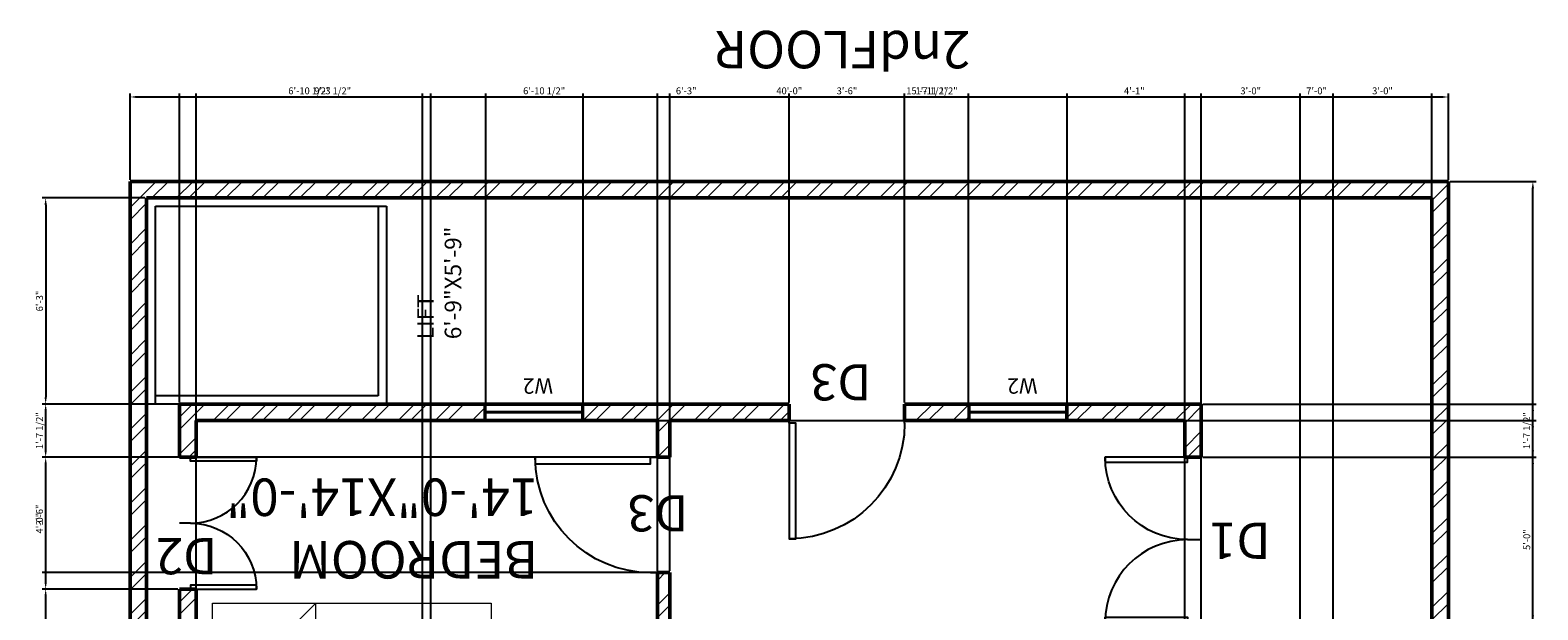
# Model space of a CAD drawing. Units: inches. Extents: x 244 to 2800, y 1060 to 1700.
# Tile 5 of 13: x 819 to 1368, y 1477 to 1688. Entities that reach past the tile are written whole.
import ezdxf

# ---------------------------------------------------------------- set-up
doc = ezdxf.new("R2010")
doc.units = ezdxf.units.IN
for name, color, linetype, lineweight in [('A-ANNO-DIMS', 2, 'Continuous', 18), ('A-ANNO-TEXT', 1, 'Continuous', 18), ('A-DOOR', 5, 'Continuous', 25), ('A-EQPM', 4, 'Continuous', 25), ('A-FURN', 9, 'Continuous', 18), ('A-GLAZ', 3, 'Continuous', 25), ('A-WALL', 7, 'Continuous', 50), ('A-WALL-PATT', 8, 'Continuous', 13)]:
    doc.layers.add(name, color=color, linetype=linetype, lineweight=lineweight)
doc.styles.get("Standard").update_dxf_attribs({"font": 'arial.ttf'})
doc.dimstyles.new('ISO-25', dxfattribs={"dimtxt": 2.5, "dimasz": 2.5, "dimexe": 1.25, "dimexo": 0.625, "dimtad": 1, "dimlunit": 4, "dimtxsty": 'Standard', "dimcen": 2.5, "dimadec": 0, "dimazin": 0, "dimtfac": 1, "dimtmove": 0, "dimatfit": 3, "dimfxl": 1, "dimarcsym": 0})

# ---------------------------------------------------------------- blocks, each defined once
blk = doc.blocks.new('*U2')
for p, q in [((0, 0), (0, -5)), ((30, 0), (30, -5))]:
    blk.add_line(p, q)
blk.add_lwpolyline([(0, 0), (0, 30), (1.75, 30), (1.75, 0)], close=True)
blk.add_arc((0, 0), 30, 0, 90)
blk = doc.blocks.new('Bed - Queen')
for p, q in [((0, -80.00003), (0, 0)), ((0, 0), (59.99999, 0)), ((59.99999, 0), (59.99999, -80.00003)), ((7.99999, -1.2), (28.79998, -1.2)), ((7.99999, -14.4), (7.99999, -1.2)), ((28.79998, -1.2), (28.79998, -14.4)), ((31.19999, -1.2), (51.99999, -1.2)), ((31.19999, -14.4), (31.19999, -1.2)), ((51.99999, -1.2), (51.99999, -16.4)), ((0, -14.4), (44.8, -14.4)), ((44.8, -16.8), (0, -16.8)), ((59.99999, -29.6), (44.8, -14.4)), ((44.8, -14.4), (44.8, -29.6)), ((51.99999, -16.4), (46.79936, -16.4)), ((44.8, -29.6), (59.99999, -29.6)), ((59.99999, -80.00003), (0, -80.00003))]:
    blk.add_line(p, q)
blk = doc.blocks.new('WIN-36')
for p, q in [((0, 0), (0, 6)), ((0, 6), (35.94, 6)), ((35.94, 6), (35.94, 0)), ((35.94, 0), (0, 0))]:
    blk.add_line(p, q)
blk = doc.blocks.new('LIFT-CAR')
for p, q in [((0, 0), (0, 72)), ((0, 72), (84, 72)), ((81, 72), (81, 3)), ((84, 72), (84, 0)), ((81, 3), (0, 3)), ((84, 0), (0, 0))]:
    blk.add_line(p, q)
blk = doc.blocks.new('*D107')
at = {"layer": 'A-ANNO-DIMS', "color": 0, "lineweight": -2, "transparency": 16777216}
for p, q in [((855.74, 1633.61), (855.74, 1664.99)), ((858.24, 1663.74), (1333.24, 1663.74)), ((1335.74, 1633.61), (1335.74, 1664.99))]:
    blk.add_line(p, q, dxfattribs=at)
at = {"layer": 'A-ANNO-DIMS', "color": 0, "transparency": 16777216}
for points in [[(858.24, 1664.15), (858.24, 1663.32), (855.74, 1663.74)], [(1333.24, 1664.15), (1333.24, 1663.32), (1335.74, 1663.74)]]:
    blk.add_solid(points, dxfattribs=at)
at = {"layer": 'Defpoints', "color": 0, "transparency": 16777216}
for p in [(1335.74, 1663.74), (855.74, 1632.99), (1335.74, 1632.99)]:
    blk.add_point(p, dxfattribs=at)
at = {"layer": 'A-ANNO-DIMS', "color": 0, "transparency": 16777216, "insert": (1095.74, 1665.64), "char_height": 2.5, "attachment_point": 5}
blk.add_mtext('40\'-0"', dxfattribs=at)
blk = doc.blocks.new('*D108')
at = {"layer": 'A-ANNO-DIMS', "color": 0, "lineweight": -2, "transparency": 16777216}
for p, q in [((1336.36, 1632.99), (1367.74, 1632.99)), ((1366.49, 1095.49), (1366.49, 1630.49)), ((1336.36, 1092.99), (1367.74, 1092.99))]:
    blk.add_line(p, q, dxfattribs=at)
at = {"layer": 'A-ANNO-DIMS', "color": 0, "transparency": 16777216}
for points in [[(1366.07, 1630.49), (1366.9, 1630.49), (1366.49, 1632.99)], [(1366.07, 1095.49), (1366.9, 1095.49), (1366.49, 1092.99)]]:
    blk.add_solid(points, dxfattribs=at)
at = {"layer": 'Defpoints', "color": 0, "transparency": 16777216}
for p in [(1335.74, 1632.99), (1366.49, 1632.99), (1335.74, 1092.99)]:
    blk.add_point(p, dxfattribs=at)
at = {"layer": 'A-ANNO-DIMS', "color": 0, "transparency": 16777216, "insert": (1364.58, 1362.99), "char_height": 2.5, "attachment_point": 5, "rotation": 90}
blk.add_mtext('45\'-0"', dxfattribs=at)
blk = doc.blocks.new('*D109')
at = {"layer": 'A-ANNO-DIMS', "color": 0, "lineweight": -2, "transparency": 16777216}
for p, q in [((861.11, 1626.99), (823.74, 1626.99)), ((824.99, 1624.49), (824.99, 1554.49)), ((873.11, 1551.99), (823.74, 1551.99))]:
    blk.add_line(p, q, dxfattribs=at)
at = {"layer": 'A-ANNO-DIMS', "color": 0, "transparency": 16777216}
for points in [[(824.57, 1624.49), (825.4, 1624.49), (824.99, 1626.99)], [(824.57, 1554.49), (825.4, 1554.49), (824.99, 1551.99)]]:
    blk.add_solid(points, dxfattribs=at)
at = {"layer": 'Defpoints', "color": 0, "transparency": 16777216}
for p in [(861.74, 1626.99), (824.99, 1551.99), (873.74, 1551.99)]:
    blk.add_point(p, dxfattribs=at)
at = {"layer": 'A-ANNO-DIMS', "color": 0, "transparency": 16777216, "insert": (823.08, 1589.49), "char_height": 2.5, "attachment_point": 5, "rotation": 90}
blk.add_mtext('6\'-3"', dxfattribs=at)
blk = doc.blocks.new('*D110')
at = {"layer": 'A-ANNO-DIMS', "color": 0, "lineweight": -2, "transparency": 16777216}
for p, q in [((1245.74, 1552.61), (1245.74, 1664.99)), ((1248.24, 1663.74), (1327.24, 1663.74)), ((1329.74, 1627.61), (1329.74, 1664.99))]:
    blk.add_line(p, q, dxfattribs=at)
at = {"layer": 'A-ANNO-DIMS', "color": 0, "transparency": 16777216}
for points in [[(1248.24, 1664.15), (1248.24, 1663.32), (1245.74, 1663.74)], [(1327.24, 1664.15), (1327.24, 1663.32), (1329.74, 1663.74)]]:
    blk.add_solid(points, dxfattribs=at)
at = {"layer": 'Defpoints', "color": 0, "transparency": 16777216}
for p in [(1329.74, 1663.74), (1329.74, 1626.99), (1245.74, 1551.99)]:
    blk.add_point(p, dxfattribs=at)
at = {"layer": 'A-ANNO-DIMS', "color": 0, "transparency": 16777216, "insert": (1287.74, 1665.64), "char_height": 2.5, "attachment_point": 5}
blk.add_mtext('7\'-0"', dxfattribs=at)
blk = doc.blocks.new('*D113')
at = {"layer": 'A-ANNO-DIMS', "color": 0, "lineweight": -2, "transparency": 16777216}
for p, q in [((873.74, 1552.61), (873.74, 1664.99)), ((876.24, 1663.74), (982.74, 1663.74)), ((985.24, 1552.61), (985.24, 1664.99))]:
    blk.add_line(p, q, dxfattribs=at)
at = {"layer": 'A-ANNO-DIMS', "color": 0, "transparency": 16777216}
for points in [[(876.24, 1664.15), (876.24, 1663.32), (873.74, 1663.74)], [(982.74, 1664.15), (982.74, 1663.32), (985.24, 1663.74)]]:
    blk.add_solid(points, dxfattribs=at)
at = {"layer": 'Defpoints', "color": 0, "transparency": 16777216}
for p in [(985.24, 1663.74), (873.74, 1551.99), (985.24, 1551.99)]:
    blk.add_point(p, dxfattribs=at)
at = {"layer": 'A-ANNO-DIMS', "color": 0, "transparency": 16777216, "insert": (929.49, 1665.65), "char_height": 2.5, "attachment_point": 5}
blk.add_mtext('9\'-3 1/2"', dxfattribs=at)
blk = doc.blocks.new('*D114')
at = {"layer": 'A-ANNO-DIMS', "color": 0, "lineweight": -2, "transparency": 16777216}
for p, q in [((1020.68, 1552.61), (1020.68, 1664.99)), ((1023.18, 1663.74), (1093.24, 1663.74)), ((1095.74, 1552.61), (1095.74, 1664.99))]:
    blk.add_line(p, q, dxfattribs=at)
at = {"layer": 'A-ANNO-DIMS', "color": 0, "transparency": 16777216}
for points in [[(1023.18, 1664.15), (1023.18, 1663.32), (1020.68, 1663.74)], [(1093.24, 1664.15), (1093.24, 1663.32), (1095.74, 1663.74)]]:
    blk.add_solid(points, dxfattribs=at)
at = {"layer": 'Defpoints', "color": 0, "transparency": 16777216}
for p in [(1095.74, 1663.74), (1020.68, 1551.99), (1095.74, 1551.99)]:
    blk.add_point(p, dxfattribs=at)
at = {"layer": 'A-ANNO-DIMS', "color": 0, "transparency": 16777216, "insert": (1058.21, 1665.64), "char_height": 2.5, "attachment_point": 5}
blk.add_mtext('6\'-3"', dxfattribs=at)
blk = doc.blocks.new('*D115')
at = {"layer": 'A-ANNO-DIMS', "color": 0, "lineweight": -2, "transparency": 16777216}
for p, q in [((1095.74, 1552.61), (1095.74, 1664.99)), ((1098.24, 1663.74), (1135.24, 1663.74)), ((1137.74, 1552.61), (1137.74, 1664.99))]:
    blk.add_line(p, q, dxfattribs=at)
at = {"layer": 'A-ANNO-DIMS', "color": 0, "transparency": 16777216}
for points in [[(1098.24, 1664.15), (1098.24, 1663.32), (1095.74, 1663.74)], [(1135.24, 1664.15), (1135.24, 1663.32), (1137.74, 1663.74)]]:
    blk.add_solid(points, dxfattribs=at)
at = {"layer": 'Defpoints', "color": 0, "transparency": 16777216}
for p in [(1137.74, 1663.74), (1095.74, 1551.99), (1137.74, 1551.99)]:
    blk.add_point(p, dxfattribs=at)
at = {"layer": 'A-ANNO-DIMS', "color": 0, "transparency": 16777216, "insert": (1116.74, 1665.64), "char_height": 2.5, "attachment_point": 5}
blk.add_mtext('3\'-6"', dxfattribs=at)
blk = doc.blocks.new('*D116')
at = {"layer": 'A-ANNO-DIMS', "color": 0, "lineweight": -2, "transparency": 16777216}
for p, q in [((1137.74, 1552.61), (1137.74, 1664.99)), ((1140.24, 1663.74), (1158.54, 1663.74)), ((1161.04, 1552.61), (1161.04, 1664.99))]:
    blk.add_line(p, q, dxfattribs=at)
at = {"layer": 'A-ANNO-DIMS', "color": 0, "transparency": 16777216}
for points in [[(1140.24, 1664.15), (1140.24, 1663.32), (1137.74, 1663.74)], [(1158.54, 1664.15), (1158.54, 1663.32), (1161.04, 1663.74)]]:
    blk.add_solid(points, dxfattribs=at)
at = {"layer": 'Defpoints', "color": 0, "transparency": 16777216}
for p in [(1161.04, 1663.74), (1137.74, 1551.99), (1161.04, 1551.99)]:
    blk.add_point(p, dxfattribs=at)
at = {"layer": 'A-ANNO-DIMS', "color": 0, "transparency": 16777216, "insert": (1149.39, 1665.65), "char_height": 2.5, "attachment_point": 5}
blk.add_mtext('1\'-11 1/2"', dxfattribs=at)
blk = doc.blocks.new('*D117')
at = {"layer": 'A-ANNO-DIMS', "color": 0, "lineweight": -2, "transparency": 16777216}
for p, q in [((1196.98, 1552.61), (1196.98, 1664.99)), ((1199.48, 1663.74), (1243.24, 1663.74)), ((1245.74, 1552.61), (1245.74, 1664.99))]:
    blk.add_line(p, q, dxfattribs=at)
at = {"layer": 'A-ANNO-DIMS', "color": 0, "transparency": 16777216}
for points in [[(1199.48, 1664.15), (1199.48, 1663.32), (1196.98, 1663.74)], [(1243.24, 1664.15), (1243.24, 1663.32), (1245.74, 1663.74)]]:
    blk.add_solid(points, dxfattribs=at)
at = {"layer": 'Defpoints', "color": 0, "transparency": 16777216}
for p in [(1245.74, 1663.74), (1196.98, 1551.99), (1245.74, 1551.99)]:
    blk.add_point(p, dxfattribs=at)
at = {"layer": 'A-ANNO-DIMS', "color": 0, "transparency": 16777216, "insert": (1221.36, 1665.62), "char_height": 2.5, "attachment_point": 5}
blk.add_mtext('4\'-1"', dxfattribs=at)
blk = doc.blocks.new('*D120')
at = {"layer": 'A-ANNO-DIMS', "color": 0, "lineweight": -2, "transparency": 16777216}
for p, q in [((873.11, 1484.64), (823.74, 1484.64)), ((824.99, 1349.76), (824.99, 1482.14)), ((873.11, 1347.26), (823.74, 1347.26))]:
    blk.add_line(p, q, dxfattribs=at)
at = {"layer": 'A-ANNO-DIMS', "color": 0, "transparency": 16777216}
for points in [[(824.57, 1482.14), (825.4, 1482.14), (824.99, 1484.64)], [(824.57, 1349.76), (825.4, 1349.76), (824.99, 1347.26)]]:
    blk.add_solid(points, dxfattribs=at)
at = {"layer": 'Defpoints', "color": 0, "transparency": 16777216}
for p in [(824.99, 1484.64), (873.74, 1484.64), (873.74, 1347.26)]:
    blk.add_point(p, dxfattribs=at)
at = {"layer": 'A-ANNO-DIMS', "color": 0, "transparency": 16777216, "insert": (823.07, 1415.95), "char_height": 2.5, "attachment_point": 5, "rotation": 90}
blk.add_mtext('11\'-5 1/2"', dxfattribs=at)
blk = doc.blocks.new('*D121')
at = {"layer": 'A-ANNO-DIMS', "color": 0, "lineweight": -2, "transparency": 16777216}
for p, q in [((873.11, 1532.64), (823.74, 1532.64)), ((824.99, 1487.14), (824.99, 1530.14)), ((873.11, 1484.64), (823.74, 1484.64))]:
    blk.add_line(p, q, dxfattribs=at)
at = {"layer": 'A-ANNO-DIMS', "color": 0, "transparency": 16777216}
for points in [[(824.57, 1530.14), (825.4, 1530.14), (824.99, 1532.64)], [(824.57, 1487.14), (825.4, 1487.14), (824.99, 1484.64)]]:
    blk.add_solid(points, dxfattribs=at)
at = {"layer": 'Defpoints', "color": 0, "transparency": 16777216}
for p in [(824.99, 1532.64), (873.74, 1532.64), (873.74, 1484.64)]:
    blk.add_point(p, dxfattribs=at)
at = {"layer": 'A-ANNO-DIMS', "color": 0, "transparency": 16777216, "insert": (823.08, 1508.64), "char_height": 2.5, "attachment_point": 5, "rotation": 90}
blk.add_mtext('4\'-0"', dxfattribs=at)
blk = doc.blocks.new('*D122')
at = {"layer": 'A-ANNO-DIMS', "color": 0, "lineweight": -2, "transparency": 16777216}
for p, q in [((873.11, 1551.99), (823.74, 1551.99)), ((824.99, 1535.14), (824.99, 1549.49)), ((873.11, 1532.64), (823.74, 1532.64))]:
    blk.add_line(p, q, dxfattribs=at)
at = {"layer": 'A-ANNO-DIMS', "color": 0, "transparency": 16777216}
for points in [[(824.57, 1549.49), (825.4, 1549.49), (824.99, 1551.99)], [(824.57, 1535.14), (825.4, 1535.14), (824.99, 1532.64)]]:
    blk.add_solid(points, dxfattribs=at)
at = {"layer": 'Defpoints', "color": 0, "transparency": 16777216}
for p in [(824.99, 1551.99), (873.74, 1551.99), (873.74, 1532.64)]:
    blk.add_point(p, dxfattribs=at)
at = {"layer": 'A-ANNO-DIMS', "color": 0, "transparency": 16777216, "insert": (823.07, 1542.31), "char_height": 2.5, "attachment_point": 5, "rotation": 90}
blk.add_mtext('1\'-7 1/2"', dxfattribs=at)
blk = doc.blocks.new('*D125')
at = {"layer": 'A-ANNO-DIMS', "color": 0, "lineweight": -2, "transparency": 16777216}
for p, q in [((880.36, 1545.99), (1367.74, 1545.99)), ((1366.49, 1375.49), (1366.49, 1543.49)), ((880.36, 1372.99), (1367.74, 1372.99))]:
    blk.add_line(p, q, dxfattribs=at)
at = {"layer": 'A-ANNO-DIMS', "color": 0, "transparency": 16777216}
for points in [[(1366.07, 1543.49), (1366.9, 1543.49), (1366.49, 1545.99)], [(1366.07, 1375.49), (1366.9, 1375.49), (1366.49, 1372.99)]]:
    blk.add_solid(points, dxfattribs=at)
at = {"layer": 'Defpoints', "color": 0, "transparency": 16777216}
for p in [(879.74, 1545.99), (1366.49, 1545.99), (879.74, 1372.99)]:
    blk.add_point(p, dxfattribs=at)
at = {"layer": 'A-ANNO-DIMS', "color": 0, "transparency": 16777216, "insert": (1364.58, 1459.49), "char_height": 2.5, "attachment_point": 5, "rotation": 90}
blk.add_mtext('14\'-5"', dxfattribs=at)
blk = doc.blocks.new('*D126')
at = {"layer": 'A-ANNO-DIMS', "color": 0, "lineweight": -2, "transparency": 16777216}
for p, q in [((879.74, 1373.61), (879.74, 1664.99)), ((882.24, 1663.74), (959.74, 1663.74)), ((962.24, 1369.11), (962.24, 1664.99))]:
    blk.add_line(p, q, dxfattribs=at)
at = {"layer": 'A-ANNO-DIMS', "color": 0, "transparency": 16777216}
for points in [[(882.24, 1664.15), (882.24, 1663.32), (879.74, 1663.74)], [(959.74, 1664.15), (959.74, 1663.32), (962.24, 1663.74)]]:
    blk.add_solid(points, dxfattribs=at)
at = {"layer": 'Defpoints', "color": 0, "transparency": 16777216}
for p in [(962.24, 1663.74), (879.74, 1372.99), (962.24, 1368.49)]:
    blk.add_point(p, dxfattribs=at)
at = {"layer": 'A-ANNO-DIMS', "color": 0, "transparency": 16777216, "insert": (920.99, 1665.65), "char_height": 2.5, "attachment_point": 5}
blk.add_mtext('6\'-10 1/2"', dxfattribs=at)
blk = doc.blocks.new('*D127')
at = {"layer": 'A-ANNO-DIMS', "color": 0, "lineweight": -2, "transparency": 16777216}
for p, q in [((965.24, 1369.11), (965.24, 1664.99)), ((967.74, 1663.74), (1045.24, 1663.74)), ((1047.74, 1373.61), (1047.74, 1664.99))]:
    blk.add_line(p, q, dxfattribs=at)
at = {"layer": 'A-ANNO-DIMS', "color": 0, "transparency": 16777216}
for points in [[(967.74, 1664.15), (967.74, 1663.32), (965.24, 1663.74)], [(1045.24, 1664.15), (1045.24, 1663.32), (1047.74, 1663.74)]]:
    blk.add_solid(points, dxfattribs=at)
at = {"layer": 'Defpoints', "color": 0, "transparency": 16777216}
for p in [(1047.74, 1663.74), (1047.74, 1372.99), (965.24, 1368.49)]:
    blk.add_point(p, dxfattribs=at)
at = {"layer": 'A-ANNO-DIMS', "color": 0, "transparency": 16777216, "insert": (1006.49, 1665.65), "char_height": 2.5, "attachment_point": 5}
blk.add_mtext('6\'-10 1/2"', dxfattribs=at)
blk = doc.blocks.new('*D138')
at = {"layer": 'A-ANNO-DIMS', "color": 0, "lineweight": -2, "transparency": 16777216}
for p, q in [((1047.11, 1532.64), (823.74, 1532.64)), ((824.99, 1493.14), (824.99, 1530.14)), ((1047.11, 1490.64), (823.74, 1490.64))]:
    blk.add_line(p, q, dxfattribs=at)
at = {"layer": 'A-ANNO-DIMS', "color": 0, "transparency": 16777216}
for points in [[(824.57, 1530.14), (825.4, 1530.14), (824.99, 1532.64)], [(824.57, 1493.14), (825.4, 1493.14), (824.99, 1490.64)]]:
    blk.add_solid(points, dxfattribs=at)
at = {"layer": 'Defpoints', "color": 0, "transparency": 16777216}
for p in [(824.99, 1532.64), (1047.74, 1532.64), (1047.74, 1490.64)]:
    blk.add_point(p, dxfattribs=at)
at = {"layer": 'A-ANNO-DIMS', "color": 0, "transparency": 16777216, "insert": (823.08, 1511.64), "char_height": 2.5, "attachment_point": 5, "rotation": 90}
blk.add_mtext('3\'-6"', dxfattribs=at)
blk = doc.blocks.new('*D141')
at = {"layer": 'A-ANNO-DIMS', "color": 0, "lineweight": -2, "transparency": 16777216}
for p, q in [((1246.36, 1532.64), (1367.74, 1532.64)), ((1366.49, 1475.14), (1366.49, 1530.14)), ((1246.36, 1472.64), (1367.74, 1472.64))]:
    blk.add_line(p, q, dxfattribs=at)
at = {"layer": 'A-ANNO-DIMS', "color": 0, "transparency": 16777216}
for points in [[(1366.07, 1530.14), (1366.9, 1530.14), (1366.49, 1532.64)], [(1366.07, 1475.14), (1366.9, 1475.14), (1366.49, 1472.64)]]:
    blk.add_solid(points, dxfattribs=at)
at = {"layer": 'Defpoints', "color": 0, "transparency": 16777216}
for p in [(1245.74, 1532.64), (1366.49, 1532.64), (1245.74, 1472.64)]:
    blk.add_point(p, dxfattribs=at)
at = {"layer": 'A-ANNO-DIMS', "color": 0, "transparency": 16777216, "insert": (1364.58, 1502.64), "char_height": 2.5, "attachment_point": 5, "rotation": 90}
blk.add_mtext('5\'-0"', dxfattribs=at)
blk = doc.blocks.new('*D142')
at = {"layer": 'A-ANNO-DIMS', "color": 0, "lineweight": -2, "transparency": 16777216}
for p, q in [((1246.36, 1551.99), (1367.74, 1551.99)), ((1366.49, 1535.14), (1366.49, 1549.49)), ((1246.36, 1532.64), (1367.74, 1532.64))]:
    blk.add_line(p, q, dxfattribs=at)
at = {"layer": 'A-ANNO-DIMS', "color": 0, "transparency": 16777216}
for points in [[(1366.07, 1549.49), (1366.9, 1549.49), (1366.49, 1551.99)], [(1366.07, 1535.14), (1366.9, 1535.14), (1366.49, 1532.64)]]:
    blk.add_solid(points, dxfattribs=at)
at = {"layer": 'Defpoints', "color": 0, "transparency": 16777216}
for p in [(1245.74, 1551.99), (1366.49, 1551.99), (1245.74, 1532.64)]:
    blk.add_point(p, dxfattribs=at)
at = {"layer": 'A-ANNO-DIMS', "color": 0, "transparency": 16777216, "insert": (1364.57, 1542.31), "char_height": 2.5, "attachment_point": 5, "rotation": 90}
blk.add_mtext('1\'-7 1/2"', dxfattribs=at)
blk = doc.blocks.new('*D145')
at = {"layer": 'A-ANNO-DIMS', "color": 0, "lineweight": -2, "transparency": 16777216}
for p, q in [((1245.74, 1243.61), (1245.74, 1664.99)), ((1248.24, 1663.74), (1279.24, 1663.74)), ((1281.74, 1243.61), (1281.74, 1664.99))]:
    blk.add_line(p, q, dxfattribs=at)
at = {"layer": 'A-ANNO-DIMS', "color": 0, "transparency": 16777216}
for points in [[(1248.24, 1664.15), (1248.24, 1663.32), (1245.74, 1663.74)], [(1279.24, 1664.15), (1279.24, 1663.32), (1281.74, 1663.74)]]:
    blk.add_solid(points, dxfattribs=at)
at = {"layer": 'Defpoints', "color": 0, "transparency": 16777216}
for p in [(1281.74, 1663.74), (1245.74, 1242.99), (1281.74, 1242.99)]:
    blk.add_point(p, dxfattribs=at)
at = {"layer": 'A-ANNO-DIMS', "color": 0, "transparency": 16777216, "insert": (1263.74, 1665.64), "char_height": 2.5, "attachment_point": 5}
blk.add_mtext('3\'-0"', dxfattribs=at)
blk = doc.blocks.new('*D146')
at = {"layer": 'A-ANNO-DIMS', "color": 0, "lineweight": -2, "transparency": 16777216}
for p, q in [((1293.74, 1243.61), (1293.74, 1664.99)), ((1296.24, 1663.74), (1327.24, 1663.74)), ((1329.74, 1243.61), (1329.74, 1664.99))]:
    blk.add_line(p, q, dxfattribs=at)
at = {"layer": 'A-ANNO-DIMS', "color": 0, "transparency": 16777216}
for points in [[(1296.24, 1664.15), (1296.24, 1663.32), (1293.74, 1663.74)], [(1327.24, 1664.15), (1327.24, 1663.32), (1329.74, 1663.74)]]:
    blk.add_solid(points, dxfattribs=at)
at = {"layer": 'Defpoints', "color": 0, "transparency": 16777216}
for p in [(1329.74, 1663.74), (1293.74, 1242.99), (1329.74, 1242.99)]:
    blk.add_point(p, dxfattribs=at)
at = {"layer": 'A-ANNO-DIMS', "color": 0, "transparency": 16777216, "insert": (1311.74, 1665.64), "char_height": 2.5, "attachment_point": 5}
blk.add_mtext('3\'-0"', dxfattribs=at)
blk = doc.blocks.new('*D147')
at = {"layer": 'A-ANNO-DIMS', "color": 0, "lineweight": -2, "transparency": 16777216}
for p, q in [((1052.24, 1491.26), (1052.24, 1664.99)), ((1054.74, 1663.74), (1237.24, 1663.74)), ((1239.74, 1473.26), (1239.74, 1664.99))]:
    blk.add_line(p, q, dxfattribs=at)
at = {"layer": 'A-ANNO-DIMS', "color": 0, "transparency": 16777216}
for points in [[(1054.74, 1664.15), (1054.74, 1663.32), (1052.24, 1663.74)], [(1237.24, 1664.15), (1237.24, 1663.32), (1239.74, 1663.74)]]:
    blk.add_solid(points, dxfattribs=at)
at = {"layer": 'Defpoints', "color": 0, "transparency": 16777216}
for p in [(1239.74, 1663.74), (1052.24, 1490.64), (1239.74, 1472.64)]:
    blk.add_point(p, dxfattribs=at)
at = {"layer": 'A-ANNO-DIMS', "color": 0, "transparency": 16777216, "insert": (1145.99, 1665.65), "char_height": 2.5, "attachment_point": 5}
blk.add_mtext('15\'-7 1/2"', dxfattribs=at)

msp = doc.modelspace()

# ---------------------------------------------------------------- hatches: boundary and pattern name
at = {"layer": 'A-WALL-PATT'}
h = msp.add_hatch(dxfattribs=at)
h.set_pattern_fill('ANSI32', color=256)
h.paths.add_polyline_path([(1335.736, 1632.986), (855.736, 1632.986), (855.736, 1092.986), (1335.736, 1092.986)])
h.paths.add_polyline_path([(1329.736, 1626.986), (1329.736, 1098.986), (1245.736, 1098.986), (861.736, 1098.986), (861.736, 1626.986)], flags=16)
h.paths.add_polyline_path([(1245.736, 1551.986), (1245.736, 1532.64), (1239.736, 1532.64), (1239.736, 1545.986), (1137.736, 1545.986), (1137.736, 1551.986)], flags=0)
h.paths.add_polyline_path([(1196.984, 1551.986), (1196.984, 1545.986), (1161.039, 1545.986), (1161.039, 1551.986)], flags=0)
h.paths.add_polyline_path([(1196.484, 1548.786), (1161.539, 1548.786), (1161.539, 1549.186), (1196.484, 1549.186)], flags=0)
h.paths.add_polyline_path([(1245.736, 1472.64), (1245.736, 1242.986), (1281.736, 1242.986), (1281.736, 1134.986), (1293.736, 1134.986), (1293.736, 1242.986), (1329.736, 1242.986), (1329.736, 1134.986), (1245.736, 1134.986), (1245.736, 1110.986), (1139.236, 1110.986), (873.736, 1110.986), (873.736, 1484.64), (879.736, 1484.64), (879.736, 1372.986), (1014.736, 1372.986), (1014.736, 1368.486), (965.236, 1368.486), (965.236, 1296.486), (1047.736, 1296.486), (1047.736, 1368.486), (1044.736, 1368.486), (1044.736, 1372.986), (1047.736, 1372.986), (1047.736, 1490.64), (1052.236, 1490.64), (1052.236, 1288.986), (1047.736, 1288.986), (1047.736, 1291.986), (912.736, 1291.986), (912.736, 1296.486), (962.236, 1296.486), (962.236, 1368.486), (879.736, 1368.486), (879.736, 1296.486), (882.736, 1296.486), (882.736, 1291.986), (879.736, 1291.986), (879.736, 1116.986), (1047.736, 1116.986), (1047.736, 1246.986), (1052.236, 1246.986), (1052.236, 1116.986), (1088.236, 1116.986), (1088.236, 1152.986), (1088.236, 1313.486), (1095.736, 1313.486), (1095.736, 1308.986), (1092.736, 1308.986), (1092.736, 1157.486), (1128.736, 1157.486), (1128.736, 1116.986), (1139.236, 1116.986), (1175.181, 1116.986), (1239.736, 1116.986), (1239.736, 1308.986), (1137.736, 1308.986), (1137.736, 1313.486), (1239.736, 1313.486), (1239.736, 1472.64)], flags=0)
h.paths.add_polyline_path([(1245.736, 1462.542), (1245.736, 1414.597), (1239.736, 1414.597), (1239.736, 1462.542)], flags=0)
h.paths.add_polyline_path([(1242.936, 1462.042), (1242.936, 1415.097), (1242.536, 1415.097), (1242.536, 1462.042)], flags=0)
h.paths.add_polyline_path([(1095.736, 1551.986), (1095.736, 1545.986), (1052.236, 1545.986), (1052.236, 1532.64), (1047.736, 1532.64), (1047.736, 1545.986), (879.736, 1545.986), (879.736, 1532.64), (873.736, 1532.64), (873.736, 1551.986), (865.04, 1551.986), (865.04, 1623.986), (949.04, 1623.986), (949.04, 1551.986)], flags=0)
h.paths.add_polyline_path([(1020.681, 1551.986), (1020.681, 1545.986), (984.736, 1545.986), (984.736, 1551.986)], flags=0)
h.paths.add_polyline_path([(1020.181, 1548.786), (985.236, 1548.786), (985.236, 1549.186), (1020.181, 1549.186)], flags=0)
h.paths.add_polyline_path([(879.736, 1347.762), (879.736, 1323.817), (873.736, 1323.817), (873.736, 1347.762)], flags=0)
h.paths.add_polyline_path([(876.936, 1347.262), (876.936, 1324.317), (876.536, 1324.317), (876.536, 1347.262)], flags=0)
h.paths.add_polyline_path([(1124.236, 1152.986), (1124.236, 1116.986), (1088.236, 1116.986), (1088.236, 1152.986)], flags=0)
h.paths.add_polyline_path([(879.736, 1287.983), (879.736, 1252.038), (873.736, 1252.038), (873.736, 1287.983)], flags=0)
h.paths.add_polyline_path([(876.936, 1287.483), (876.936, 1252.538), (876.536, 1252.538), (876.536, 1287.483)], flags=0)
h.paths.add_polyline_path([(1175.181, 1116.986), (1175.181, 1110.986), (1139.236, 1110.986), (1139.236, 1114.186), (1174.681, 1114.186), (1174.681, 1116.986)], flags=0)
h.paths.add_polyline_path([(1040.103, 1116.986), (1040.103, 1110.986), (1004.158, 1110.986), (1004.158, 1116.986)], flags=0)
h.paths.add_polyline_path([(1039.603, 1113.786), (1004.658, 1113.786), (1004.658, 1114.186), (1039.603, 1114.186)], flags=0)
h.paths.add_polyline_path([(1164.972, 1113.308), (1150.368, 1113.308), (1150.368, 1101.713), (1164.972, 1101.713)], flags=8)
h.paths.add_polyline_path([(1033.179, 1112.552), (1018.576, 1112.552), (1018.576, 1100.958), (1033.179, 1100.958)], flags=8)
h.paths.add_polyline_path([(874.571, 1270.316), (859.967, 1270.316), (859.967, 1258.722), (874.571, 1258.722)], flags=24)
h.paths.add_polyline_path([(1011.225, 1564.465), (996.622, 1564.465), (996.622, 1552.871), (1011.225, 1552.871)], flags=8)
h.paths.add_polyline_path([(1187.63, 1564.482), (1173.026, 1564.482), (1173.026, 1552.887), (1187.63, 1552.887)], flags=8)
h.paths.add_polyline_path([(1259.132, 1444.47), (1244.529, 1444.47), (1244.529, 1432.875), (1259.132, 1432.875)], flags=8)
h.paths.add_polyline_path([(875.239, 1344.511), (860.635, 1344.511), (860.635, 1332.916), (875.239, 1332.916)], flags=24)
h.paths.add_polyline_path([(892.18, 1510.489), (862.03, 1510.489), (862.03, 1483.307), (892.18, 1483.307)], flags=8)
h.paths.add_polyline_path([(912.199, 1310.068), (882.049, 1310.068), (882.049, 1282.887), (912.199, 1282.887)], flags=8)
h.paths.add_polyline_path([(1043.03, 1389.229), (1012.88, 1389.229), (1012.88, 1362.047), (1043.03, 1362.047)], flags=8)
h.paths.add_polyline_path([(1058.3, 1285.41), (1028.149, 1285.41), (1028.149, 1258.229), (1058.3, 1258.229)], flags=8)
h.paths.add_polyline_path([(1129.051, 1325.331), (1098.901, 1325.331), (1098.901, 1298.15), (1129.051, 1298.15)], flags=8)
h.paths.add_polyline_path([(1063.761, 1526.078), (1033.611, 1526.078), (1033.611, 1498.897), (1063.761, 1498.897)], flags=8)
h.paths.add_polyline_path([(1130.374, 1573.756), (1100.224, 1573.756), (1100.224, 1546.575), (1130.374, 1546.575)], flags=8)
h.paths.add_polyline_path([(1275.672, 1516.103), (1245.522, 1516.103), (1245.522, 1488.922), (1275.672, 1488.922)], flags=8)
h.paths.add_polyline_path([(979.613, 1573.477), (979.613, 1615.869), (957.159, 1615.869), (957.159, 1573.477)], flags=8)
h.paths.add_polyline_path([(1311.481, 1266.003), (1254.484, 1266.003), (1254.484, 1252.05), (1311.481, 1252.05)], flags=8)
h.paths.add_polyline_path([(1159.757, 1266.713), (1159.757, 1153.038), (1197.594, 1153.038), (1197.594, 1266.713)], flags=8)
h.paths.add_polyline_path([(1139.055, 1456.095), (1139.055, 1323.863), (1184.409, 1323.863), (1184.409, 1456.095)], flags=8)
h.paths.add_polyline_path([(936.318, 1364.302), (878.595, 1364.302), (878.595, 1333.511), (936.318, 1333.511)], flags=8)
h.paths.add_polyline_path([(1042.961, 1335.109), (985.238, 1335.109), (985.238, 1304.318), (1042.961, 1304.318)], flags=8)
h.paths.add_polyline_path([(1002.135, 1273.839), (885.452, 1273.839), (885.452, 1222.91), (1002.135, 1222.91)], flags=8)
h.paths.add_polyline_path([(1009.771, 1532.646), (893.088, 1532.646), (893.088, 1481.717), (1009.771, 1481.717)], flags=8)
h = msp.add_hatch(dxfattribs=at)
h.set_pattern_fill('ANSI32', color=256)
h.paths.add_polyline_path([(984.736, 1551.986), (873.736, 1551.986), (873.736, 1532.64), (877.736, 1532.64), (879.736, 1532.64), (879.736, 1545.986), (984.736, 1545.986)])
h = msp.add_hatch(dxfattribs=at)
h.set_pattern_fill('ANSI32', color=256)
h.paths.add_polyline_path([(1095.736, 1551.986), (1055.236, 1551.986), (1020.681, 1551.986), (1020.681, 1545.986), (1047.736, 1545.986), (1047.736, 1532.64), (1052.236, 1532.64), (1052.236, 1545.986), (1055.236, 1545.986), (1095.736, 1545.986)])
h = msp.add_hatch(dxfattribs=at)
h.set_pattern_fill('ANSI32', color=256)
h.paths.add_polyline_path([(1161.039, 1551.986), (1137.736, 1551.986), (1137.736, 1545.986), (1161.039, 1545.986)])
h = msp.add_hatch(dxfattribs=at)
h.set_pattern_fill('ANSI32', color=256)
h.paths.add_polyline_path([(1245.736, 1551.986), (1196.984, 1551.986), (1196.984, 1545.986), (1239.736, 1545.986), (1239.736, 1532.64), (1245.736, 1532.64)])
h = msp.add_hatch(dxfattribs=at)
h.set_pattern_fill('ANSI32', color=256)
h.paths.add_polyline_path([(1052.236, 1490.64), (1047.736, 1490.64), (1047.736, 1372.986), (1044.736, 1372.986), (1044.736, 1368.486), (1047.736, 1368.486), (1047.736, 1296.486), (965.236, 1296.486), (965.236, 1368.486), (1014.736, 1368.486), (1014.736, 1372.986), (879.736, 1372.986), (879.736, 1484.64), (877.736, 1484.64), (873.736, 1484.64), (873.736, 1347.762), (879.736, 1347.762), (879.736, 1368.486), (962.236, 1368.486), (962.236, 1296.486), (912.736, 1296.486), (912.736, 1291.986), (915.736, 1291.986), (1047.736, 1291.986), (1047.736, 1288.986), (1052.236, 1288.986)])

# ---------------------------------------------------------------- linework, layer by layer
at = {"layer": 'A-GLAZ'}
for p, q in [((985.236, 1545.986), (985.236, 1551.986)), ((1020.181, 1549.186), (985.236, 1549.186)), ((1020.181, 1548.786), (985.236, 1548.786)), ((1020.181, 1551.986), (1020.181, 1545.986)), ((1161.539, 1545.986), (1161.539, 1551.986)), ((1196.484, 1549.186), (1161.539, 1549.186)), ((1196.484, 1548.786), (1161.539, 1548.786)), ((1196.484, 1551.986), (1196.484, 1545.986))]:
    msp.add_line(p, q, dxfattribs=at)
at = {"layer": 'A-WALL'}
for p, q in [((1335.736, 1632.986), (855.736, 1632.986)), ((855.736, 1632.986), (855.736, 1092.986)), ((1335.736, 1092.986), (1335.736, 1632.986)), ((1329.736, 1626.986), (861.736, 1626.986)), ((861.736, 1626.986), (861.736, 1098.986)), ((1329.736, 1098.986), (1329.736, 1626.986)), ((873.736, 1551.986), (873.736, 1532.64)), ((873.736, 1551.986), (1095.736, 1551.986)), ((1055.236, 1551.986), (1095.736, 1551.986)), ((1095.736, 1545.986), (1095.736, 1551.986)), ((1137.736, 1551.986), (1245.736, 1551.986)), ((1137.736, 1551.986), (1137.736, 1545.986)), ((1245.736, 1532.64), (1245.736, 1551.986)), ((879.736, 1545.986), (879.736, 1532.64)), ((879.736, 1545.986), (1047.736, 1545.986)), ((1047.736, 1545.986), (1047.736, 1532.64)), ((1052.236, 1545.986), (1052.236, 1532.64)), ((1052.236, 1545.986), (1095.736, 1545.986)), ((1052.236, 1545.986), (1055.236, 1545.986)), ((1137.736, 1545.986), (1239.736, 1545.986)), ((1239.736, 1532.64), (1239.736, 1545.986)), ((879.736, 1532.64), (873.736, 1532.64)), ((1052.236, 1532.64), (1047.736, 1532.64)), ((1239.657, 1532.64), (1245.736, 1532.64)), ((1047.736, 1490.64), (1047.736, 1372.986)), ((1047.736, 1490.64), (1052.236, 1490.64)), ((1052.236, 1490.64), (1052.236, 1288.986)), ((873.736, 1484.64), (879.736, 1484.64)), ((873.736, 1484.64), (873.736, 1110.986)), ((879.736, 1484.64), (879.736, 1372.986))]:
    msp.add_line(p, q, dxfattribs=at)

# ---------------------------------------------------------------- block references
at = {"layer": 'A-DOOR'}
for p, xscale, yscale, zscale, rotation in [((1095.736, 1544.986), -1.399999999999999, 1.399999999999999, 1.399999999999999, 180), ((877.736, 1532.64), 0.8000000000000049, 0.8000000000000049, 0.8000000000000049, 270), ((1045.236, 1532.64), -1.399999999999999, 1.399999999999999, 1.399999999999999, 90), ((1240.736, 1532.64), -0.9999956819955501, 0.9999956819955501, 0.9999956819955501, 90), ((877.736, 1484.64), -0.8000000000000049, 0.8000000000000049, 0.8000000000000049, 270), ((1240.736, 1472.64), 0.9999956819955501, 0.9999956819955501, 0.9999956819955501, 90)]:
    msp.add_blockref('*U2', p, dxfattribs=dict(at, xscale=xscale, yscale=yscale, zscale=zscale, rotation=rotation))
at = {"layer": 'A-EQPM'}
msp.add_blockref('LIFT-CAR', (865.04, 1551.986), dxfattribs=at)
at = {"layer": 'A-FURN', "xscale": 1.268227082860182, "yscale": 1.268227082860182, "zscale": 1.268227082860182, "rotation": 90}
msp.add_blockref('Bed - Queen', (885.782, 1403.45), dxfattribs=at)
at = {"layer": 'A-GLAZ', "rotation": 180}
for p in [(1020.681, 1551.986), (1196.984, 1551.986)]:
    msp.add_blockref('WIN-36', p, dxfattribs=at)

# ---------------------------------------------------------------- texts
at = {"layer": 'A-ANNO-TEXT', "attachment_point": 1}
for s, width, gutter_width, insert, char_height, rotation in [('2ndFLOOR', 25.27039, 68.243, (1161.668, 1674.165), 13.6485, 180), ('LIFT\\P6\'-9"X5\'-9"', 12.02436, 30.086, (960.256, 1575.597), 6.01727, 90), ('D3', 20.58737, 65.951, (1125.655, 1553.309), 13.1902, 180), ('W2', 2.91536, 28.132, (1009.723, 1555.743), 5.6265, 180), ('W2', 2.91536, 28.132, (1186.127, 1555.76), 5.6265, 180), ('BEDROOM\\P14\'-0"X14\'-0"', 25.27039, 68.243, (1004.282, 1488.499), 13.64851, 180), ('D3', 20.58737, 65.951, (1059.042, 1505.631), 13.1902, 180), ('D1', 20.58737, 65.951, (1270.953, 1495.656), 13.1902, 180), ('D2', 20.58737, 65.951, (887.461, 1490.042), 13.1902, 180)]:
    msp.add_mtext_dynamic_manual_height_columns(s, width=width, gutter_width=gutter_width, heights=[0], dxfattribs=dict(at, insert=insert, char_height=char_height, rotation=rotation))

# ---------------------------------------------------------------- dimensions: what is measured, and where the dimension line sits
at = {"layer": 'A-ANNO-DIMS'}
for base, p1, p2, picture, middle in [((985.236, 1663.736), (873.736, 1551.986), (985.236, 1551.986), '*D113', (929.486, 1665.655)), ((962.236, 1663.736), (879.736, 1372.986), (962.236, 1368.486), '*D126', (920.986, 1665.654)), ((1047.736, 1663.736), (965.236, 1368.486), (1047.736, 1372.986), '*D127', (1006.486, 1665.654)), ((1239.736, 1663.736), (1052.236, 1490.64), (1239.736, 1472.64), '*D147', (1145.986, 1665.654)), ((1161.039, 1663.736), (1137.736, 1551.986), (1161.039, 1551.986), '*D116', (1149.388, 1665.654)), ((1335.736, 1663.736), (855.736, 1632.986), (1335.736, 1632.986), '*D107', (1095.736, 1665.638)), ((1095.736, 1663.736), (1020.681, 1551.986), (1095.736, 1551.986), '*D114', (1058.208, 1665.638)), ((1137.736, 1663.736), (1095.736, 1551.986), (1137.736, 1551.986), '*D115', (1116.736, 1665.638)), ((1245.736, 1663.736), (1196.984, 1551.986), (1245.736, 1551.986), '*D117', (1221.36, 1665.616)), ((1281.736, 1663.736), (1245.736, 1242.986), (1281.736, 1242.986), '*D145', (1263.736, 1665.638)), ((1329.736, 1663.736), (1245.736, 1551.986), (1329.736, 1626.986), '*D110', (1287.736, 1665.638)), ((1329.736, 1663.736), (1293.736, 1242.986), (1329.736, 1242.986), '*D146', (1311.736, 1665.638))]:
    dim = msp.add_linear_dim(base=base, p1=p1, p2=p2, dimstyle='ISO-25', override={"dimdec": 1, "dimlfac": 1, "dimrnd": 0, "dimzin": 1, "dimdsep": 46, "dimlunit": 4, "dimfrac": 2}, dxfattribs=at)
    dim.commit()
    dim.dimension.update_dxf_attribs({"geometry": picture, "text_midpoint": middle})
for base, p1, p2, picture, middle in [((1366.486, 1632.986), (1335.736, 1092.986), (1335.736, 1632.986), '*D108', (1364.585, 1362.986)), ((824.986, 1551.986), (861.736, 1626.986), (873.736, 1551.986), '*D109', (823.084, 1589.486)), ((824.986, 1551.986), (873.736, 1532.64), (873.736, 1551.986), '*D122', (823.068, 1542.313)), ((1366.486, 1551.986), (1245.736, 1532.64), (1245.736, 1551.986), '*D142', (1364.568, 1542.313)), ((1366.486, 1545.986), (879.736, 1372.986), (879.736, 1545.986), '*D125', (1364.585, 1459.486)), ((824.986, 1532.64), (1047.736, 1490.64), (1047.736, 1532.64), '*D138', (823.084, 1511.64)), ((824.986, 1532.64), (873.736, 1484.64), (873.736, 1532.64), '*D121', (823.085, 1508.64)), ((1366.486, 1532.64), (1245.736, 1472.64), (1245.736, 1532.64), '*D141', (1364.585, 1502.64)), ((824.986, 1484.64), (873.736, 1347.262), (873.736, 1484.64), '*D120', (823.068, 1415.951))]:
    dim = msp.add_linear_dim(base=base, p1=p1, p2=p2, angle=90, dimstyle='ISO-25', override={"dimdec": 1, "dimlfac": 1, "dimrnd": 0, "dimzin": 1, "dimdsep": 46, "dimlunit": 4, "dimfrac": 2}, dxfattribs=at)
    dim.commit()
    dim.dimension.update_dxf_attribs({"geometry": picture, "text_midpoint": middle})

doc.saveas('drawing.dxf')
